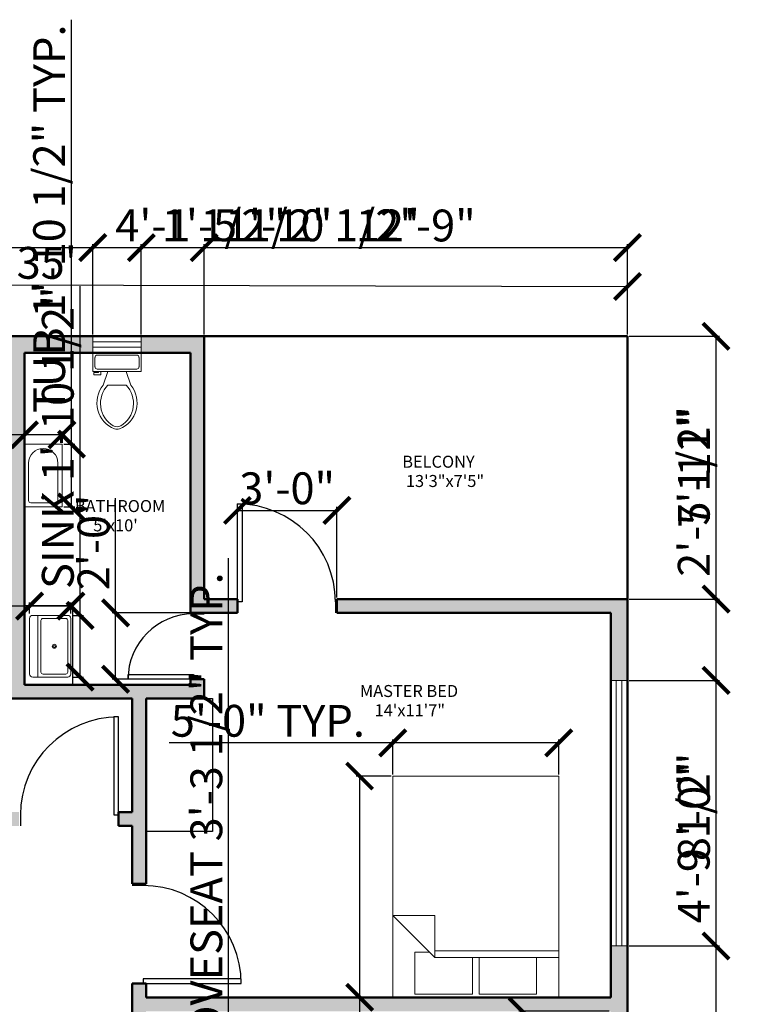
# Model space of a CAD drawing. Units: inches. Extents: x 3147 to 3847, y 1414 to 2207.
# Tile 7 of 7: x 3550 to 3812, y 1852 to 2207. Entities that reach past the tile are written whole.
import ezdxf

# ---------------------------------------------------------------- set-up
doc = ezdxf.new("R2010")
doc.units = ezdxf.units.IN
for name, color, linetype, lineweight in [('A-ANNO-DIMS', 2, 'Continuous', 18), ('A-AREA-IDEN', 7, 'Continuous', 18), ('A-DOOR', 3, 'Continuous', 25), ('A-FLOR-CASE', 32, 'Continuous', 25), ('A-FLOR-FIXT', 9, 'Continuous', 18), ('A-FURN', 8, 'Continuous', 18), ('A-GLAZ', 4, 'Continuous', 18), ('A-WALL', 7, 'Continuous', 50)]:
    doc.layers.add(name, color=color, linetype=linetype, lineweight=lineweight)
doc.layers.add('A-WALL-PATT', color=18, linetype='Continuous', lineweight=13, true_color=0x000000)
doc.styles.get("Standard").update_dxf_attribs({"font": 'arial.ttf'})
doc.dimstyles.new('ISO-25', dxfattribs={"dimtxt": 11.5, "dimasz": 9.5, "dimexe": 1.25, "dimexo": 0.625, "dimtad": 1, "dimdec": 0, "dimlunit": 3, "dimtxsty": 'Standard', "dimblk": 'ARCHTICK', "dimcen": 2.5, "dimadec": 0, "dimazin": 0, "dimtfac": 1, "dimtdec": 0, "dimtmove": 0, "dimatfit": 3, "dimfxl": 1, "dimarcsym": 0})

# ---------------------------------------------------------------- blocks, each defined once
blk = doc.blocks.new('*U6')
for p, q in [((0, 0), (0, -100)), ((900, 0), (900, -100))]:
    blk.add_line(p, q)
blk.add_lwpolyline([(0, 0), (0, 900), (43.75, 900), (43.75, 0)], close=True)
blk.add_arc((0, 0), 900, 0, 90)
blk = doc.blocks.new('*U5')
for p, q in [((0, 0), (0, -100)), ((-900, 0), (-900, -100))]:
    blk.add_line(p, q)
blk.add_lwpolyline([(0, 0), (0, 900), (-43.75, 900), (-43.75, 0)], close=True)
blk.add_arc((0, 0), 900, 90, 180)
blk = doc.blocks.new('*U7')
for p, q in [((0, 0), (0, -100)), ((600, 0), (600, -100))]:
    blk.add_line(p, q)
blk.add_lwpolyline([(0, 0), (0, 600), (43.75, 600), (43.75, 0)], close=True)
blk.add_arc((0, 0), 600, 0, 90)
blk = doc.blocks.new('Bed - Queen')
for p, q in [((0, -80.00003), (0, 0)), ((0, 0), (59.99999, 0)), ((59.99999, 0), (59.99999, -80.00003)), ((7.99999, -1.2), (28.79998, -1.2)), ((7.99999, -14.4), (7.99999, -1.2)), ((28.79998, -1.2), (28.79998, -14.4)), ((31.19999, -1.2), (51.99999, -1.2)), ((31.19999, -14.4), (31.19999, -1.2)), ((51.99999, -1.2), (51.99999, -16.4)), ((0, -14.4), (44.8, -14.4)), ((44.8, -16.8), (0, -16.8)), ((59.99999, -29.6), (44.8, -14.4)), ((44.8, -14.4), (44.8, -29.6)), ((51.99999, -16.4), (46.79936, -16.4)), ((44.8, -29.6), (59.99999, -29.6)), ((59.99999, -80.00003), (0, -80.00003))]:
    blk.add_line(p, q)
blk = doc.blocks.new('Sink-single - 30 in top')
blk.add_line((-15, -3.999996), (15, -3.999996))
for points in [[(-13.5, 0), (13.5, 0)], [(-15, -18.499996), (-15, -1.5)], [(15, -1.5), (15, -18.499996)], [(-13.5, -17.499996), (-13.5, -6.499996)], [(-12.5, -5.499996), (12.5, -5.499996)], [(13.5, -6.499996), (13.5, -17.499996)], [(12.5, -18.499996), (-12.5, -18.499996)], [(13.5, -19.999996), (-13.5, -19.999996)]]:
    blk.add_lwpolyline(points)
for radius in [1, 0.5]:
    blk.add_circle((0, -11.999996), radius)
for centre, radius, start, end in [((-13.5, -1.5), 1.5, 90, 180), ((13.5, -1.5), 1.5, 0, 90), ((-12.5, -6.499996), 1, 90, 180), ((12.5, -6.499996), 1, 0, 90), ((-13.5, -18.499996), 1.5, 180, 270), ((-12.5, -17.499996), 1, 180, 270), ((12.5, -17.499996), 1, 270, 0), ((13.5, -18.499996), 1.5, 270, 0)]:
    blk.add_arc(centre, radius, start, end)
blk = doc.blocks.new('Toilet - top')
for p, q in [((9.5, -6), (9.5, -2)), ((-10, -8.5), (-8, -8.5)), ((-10, -9.5), (-10, -8.5)), ((-8, -8.5), (-8, -8)), ((-7, -8), (-7, -9.5)), ((-4, -8), (-6, -14)), ((4, -8), (6, -14)), ((-7, -9.5), (-10, -9.5)), ((4, -14), (-4, -14))]:
    blk.add_line(p, q)
blk.add_lwpolyline([(10.5, -8), (10.5, 0), (-10.5, 0), (-10.5, -8)], close=True)
for points in [[(-9.5, -2), (-9.5, -6)], [(8.5, -1), (-8.5, -1)], [(-8.5, -7), (8.5, -7)]]:
    blk.add_lwpolyline(points)
for centre, radius, start, end in [((-8.62, -1.88), 0.884, 81.8699, 188.1301), ((8.62, -1.88), 0.884, 351.8699, 98.1301), ((-8.62, -6.12), 0.884, 171.8699, 278.1301), ((8.62, -6.12), 0.884, 261.8699, 8.1301), ((3.52, -21.58), 12.17, 141.4691, 247.9714), ((4.2, -21.82), 11.33, 136.3677, 238.9468), ((-3.52, -21.58), 12.17, 292.0284, 38.5307), ((-4.2, -21.82), 11.33, 301.053, 43.6321), ((0, -27.88), 4, 245.7318, 294.2682), ((0, -29), 4, 254.8605, 285.1395)]:
    blk.add_arc(centre, radius, start, end)
blk = doc.blocks.new('Bath Tub - 26 x 60 in.')
for p, q in [((8, -18), (10, -18)), ((9, -17), (9, -19))]:
    blk.add_line(p, q)
blk.add_lwpolyline([(0, -36), (0, 0), (60, 0), (60, -36)], close=True)
for points in [[(4, -30), (4, -6)], [(6, -4), (42, -4)], [(42, -32), (6, -32)]]:
    blk.add_lwpolyline(points)
for radius in [1.5, 1]:
    blk.add_circle((9, -18), radius)
for centre, radius, start, end in [((5.75, -5.75), 1.77, 81.8699, 188.1301), ((42, -18), 14, 270, 90), ((5.75, -30.25), 1.77, 171.8699, 278.1301)]:
    blk.add_arc(centre, radius, start, end)
blk = doc.blocks.new('_ArchTick')
at = {"color": 0, "linetype": 'ByBlock', "const_width": 0.15}
blk.add_lwpolyline([(-0.5, -0.5), (0.5, 0.5)], dxfattribs=at)
blk = doc.blocks.new('*D23')
at = {"layer": 'A-ANNO-DIMS', "color": 0, "lineweight": -2, "transparency": 16777216}
for p, q in [((3349.77, 2094.75), (3349.81, 2113.37)), ((3349.81, 2112.12), (3769.81, 2111.04)), ((3769.77, 2093.67), (3769.81, 2112.29))]:
    blk.add_line(p, q, dxfattribs=at)
at = {"layer": 'Defpoints', "color": 0, "transparency": 16777216}
for p in [(3769.81, 2111.04), (3349.76, 2094.13), (3769.76, 2093.05)]:
    blk.add_point(p, dxfattribs=at)
at = {"layer": 'A-ANNO-DIMS', "color": 0, "lineweight": -2, "transparency": 16777216, "xscale": 9.5, "yscale": 9.5, "zscale": 9.5}
for p, rotation in [((3349.81, 2112.12), 179.8528346034433), ((3769.81, 2111.04), 359.8528346034433)]:
    blk.add_blockref('_ArchTick', p, dxfattribs=dict(at, rotation=rotation))
at = {"layer": 'A-ANNO-DIMS', "color": 0, "transparency": 16777216, "insert": (3559.83, 2118.08), "char_height": 11.5, "attachment_point": 5, "rotation": 359.8528}
blk.add_mtext("35'", dxfattribs=at)
blk = doc.blocks.new('*D29')
at = {"layer": 'A-ANNO-DIMS', "color": 0, "lineweight": -2, "transparency": 16777216}
for p, q in [((3568.76, 2054.03), (3568.76, 2207.49)), ((3565.99, 2054.03), (3570.01, 2054.03)), ((3568.76, 2031.36), (3568.76, 2054.03)), ((3565.99, 2031.36), (3570.01, 2031.36))]:
    blk.add_line(p, q, dxfattribs=at)
at = {"layer": 'Defpoints', "color": 0, "transparency": 16777216}
for p in [(3565.36, 2054.03), (3568.76, 2054.03), (3565.36, 2031.36)]:
    blk.add_point(p, dxfattribs=at)
at = {"layer": 'A-ANNO-DIMS', "color": 0, "lineweight": -2, "transparency": 16777216, "xscale": 9.5, "yscale": 9.5, "zscale": 9.5}
for p, rotation in [((3568.76, 2054.03), 90), ((3568.76, 2031.36), 270)]:
    blk.add_blockref('_ArchTick', p, dxfattribs=dict(at, rotation=rotation))
at = {"layer": 'A-ANNO-DIMS', "color": 0, "transparency": 16777216, "insert": (3562.19, 2135.51), "char_height": 11.5, "attachment_point": 5, "rotation": 90}
blk.add_mtext('TUB 1\'-10 1/2" TYP.', dxfattribs=at)
blk = doc.blocks.new('*D30')
at = {"layer": 'A-ANNO-DIMS', "color": 0, "lineweight": -2, "transparency": 16777216}
for p, q in [((3551.76, 2057.43), (3445.2, 2057.43)), ((3551.76, 2054.65), (3551.76, 2058.68)), ((3565.36, 2057.43), (3551.76, 2057.43)), ((3565.36, 2054.65), (3565.36, 2058.68))]:
    blk.add_line(p, q, dxfattribs=at)
at = {"layer": 'Defpoints', "color": 0, "transparency": 16777216}
for p in [(3551.76, 2057.43), (3551.76, 2054.03), (3565.36, 2054.03)]:
    blk.add_point(p, dxfattribs=at)
at = {"layer": 'A-ANNO-DIMS', "color": 0, "lineweight": -2, "transparency": 16777216, "xscale": 9.5, "yscale": 9.5, "zscale": 9.5, "rotation": 180}
blk.add_blockref('_ArchTick', (3551.76, 2057.43), dxfattribs=at)
at = {"layer": 'A-ANNO-DIMS', "color": 0, "lineweight": -2, "transparency": 16777216, "xscale": 9.5, "yscale": 9.5, "zscale": 9.5}
blk.add_blockref('_ArchTick', (3565.36, 2057.43), dxfattribs=at)
at = {"layer": 'A-ANNO-DIMS', "color": 0, "transparency": 16777216, "insert": (3493.73, 2064), "char_height": 11.5, "attachment_point": 5}
blk.add_mtext('1\'-1 1/2" TYP.', dxfattribs=at)
blk = doc.blocks.new('*D33')
at = {"layer": 'A-ANNO-DIMS', "color": 0, "lineweight": -2, "transparency": 16777216}
for p, q in [((3684.32, 1934.05), (3671.7, 1934.05)), ((3672.95, 1934.05), (3672.95, 1854.05)), ((3684.32, 1854.05), (3671.7, 1854.05)), ((3672.95, 1854.05), (3672.95, 1736.21))]:
    blk.add_line(p, q, dxfattribs=at)
at = {"layer": 'Defpoints', "color": 0, "transparency": 16777216}
for p in [(3684.95, 1934.05), (3672.95, 1854.05), (3684.95, 1854.05)]:
    blk.add_point(p, dxfattribs=at)
at = {"layer": 'A-ANNO-DIMS', "color": 0, "lineweight": -2, "transparency": 16777216, "xscale": 9.5, "yscale": 9.5, "zscale": 9.5}
for p, rotation in [((3672.95, 1934.05), 90), ((3672.95, 1854.05), 270)]:
    blk.add_blockref('_ArchTick', p, dxfattribs=dict(at, rotation=rotation))
at = {"layer": 'A-ANNO-DIMS', "color": 0, "transparency": 16777216, "insert": (3666.45, 1790.38), "char_height": 11.5, "attachment_point": 5, "rotation": 90}
blk.add_mtext('BED 6\'-8" TYP.', dxfattribs=at)
blk = doc.blocks.new('*D34')
at = {"layer": 'A-ANNO-DIMS', "color": 0, "lineweight": -2, "transparency": 16777216}
for p, q in [((3684.95, 1934.67), (3684.95, 1947.3)), ((3744.95, 1934.67), (3744.95, 1947.3)), ((3684.95, 1946.05), (3604.1, 1946.05)), ((3744.95, 1946.05), (3684.95, 1946.05))]:
    blk.add_line(p, q, dxfattribs=at)
at = {"layer": 'Defpoints', "color": 0, "transparency": 16777216}
for p in [(3684.95, 1946.05), (3684.95, 1934.05), (3744.95, 1934.05)]:
    blk.add_point(p, dxfattribs=at)
at = {"layer": 'A-ANNO-DIMS', "color": 0, "lineweight": -2, "transparency": 16777216, "xscale": 9.5, "yscale": 9.5, "zscale": 9.5, "rotation": 180}
blk.add_blockref('_ArchTick', (3684.95, 1946.05), dxfattribs=at)
at = {"layer": 'A-ANNO-DIMS', "color": 0, "lineweight": -2, "transparency": 16777216, "xscale": 9.5, "yscale": 9.5, "zscale": 9.5}
blk.add_blockref('_ArchTick', (3744.95, 1946.05), dxfattribs=at)
at = {"layer": 'A-ANNO-DIMS', "color": 0, "transparency": 16777216, "insert": (3639.78, 1952.55), "char_height": 11.5, "attachment_point": 5}
blk.add_mtext('5\'-0" TYP.', dxfattribs=at)
blk = doc.blocks.new('*D37')
at = {"layer": 'A-ANNO-DIMS', "color": 0, "lineweight": -2, "transparency": 16777216}
for p, q in [((3625.6, 1816.38), (3625.6, 2012.8)), ((3620.32, 1816.38), (3626.85, 1816.38)), ((3625.6, 1777.02), (3625.6, 1816.38)), ((3620.32, 1777.02), (3626.85, 1777.02))]:
    blk.add_line(p, q, dxfattribs=at)
at = {"layer": 'Defpoints', "color": 0, "transparency": 16777216}
for p in [(3619.7, 1816.38), (3625.6, 1816.38), (3619.7, 1777.02)]:
    blk.add_point(p, dxfattribs=at)
at = {"layer": 'A-ANNO-DIMS', "color": 0, "lineweight": -2, "transparency": 16777216, "xscale": 9.5, "yscale": 9.5, "zscale": 9.5}
for p, rotation in [((3625.6, 1816.38), 90), ((3625.6, 1777.02), 270)]:
    blk.add_blockref('_ArchTick', p, dxfattribs=dict(at, rotation=rotation))
at = {"layer": 'A-ANNO-DIMS', "color": 0, "transparency": 16777216, "insert": (3619.02, 1919.34), "char_height": 11.5, "attachment_point": 5, "rotation": 90}
blk.add_mtext('LOVESEAT 3\'-3 1/2" TYP.', dxfattribs=at)
blk = doc.blocks.new('*D47')
at = {"layer": 'A-ANNO-DIMS', "color": 0, "lineweight": -2, "transparency": 16777216}
for p, q in [((3571.89, 1992.16), (3571.89, 2111.11)), ((3569.17, 1992.16), (3573.14, 1992.16)), ((3571.89, 1969.81), (3571.89, 1992.16)), ((3569.17, 1969.81), (3573.14, 1969.81))]:
    blk.add_line(p, q, dxfattribs=at)
at = {"layer": 'Defpoints', "color": 0, "transparency": 16777216}
for p in [(3568.54, 1992.16), (3571.89, 1992.16), (3568.54, 1969.81)]:
    blk.add_point(p, dxfattribs=at)
at = {"layer": 'A-ANNO-DIMS', "color": 0, "lineweight": -2, "transparency": 16777216, "xscale": 9.5, "yscale": 9.5, "zscale": 9.5}
for p, rotation in [((3571.89, 1992.16), 90), ((3571.89, 1969.81), 270)]:
    blk.add_blockref('_ArchTick', p, dxfattribs=dict(at, rotation=rotation))
at = {"layer": 'A-ANNO-DIMS', "color": 0, "transparency": 16777216, "insert": (3565.32, 2056.38), "char_height": 11.5, "attachment_point": 5, "rotation": 90}
blk.add_mtext('SINK 1\'-10 1/2"', dxfattribs=at)
blk = doc.blocks.new('*D48')
at = {"layer": 'A-ANNO-DIMS', "color": 0, "lineweight": -2, "transparency": 16777216}
for p, q in [((3553.64, 1995.51), (3513.41, 1995.51)), ((3553.64, 1992.78), (3553.64, 1996.76)), ((3568.54, 1995.51), (3553.64, 1995.51)), ((3568.54, 1992.78), (3568.54, 1996.76))]:
    blk.add_line(p, q, dxfattribs=at)
at = {"layer": 'Defpoints', "color": 0, "transparency": 16777216}
for p in [(3553.64, 1995.51), (3553.64, 1992.16), (3568.54, 1992.16)]:
    blk.add_point(p, dxfattribs=at)
at = {"layer": 'A-ANNO-DIMS', "color": 0, "lineweight": -2, "transparency": 16777216, "xscale": 9.5, "yscale": 9.5, "zscale": 9.5, "rotation": 180}
blk.add_blockref('_ArchTick', (3553.64, 1995.51), dxfattribs=at)
at = {"layer": 'A-ANNO-DIMS', "color": 0, "lineweight": -2, "transparency": 16777216, "xscale": 9.5, "yscale": 9.5, "zscale": 9.5}
blk.add_blockref('_ArchTick', (3568.54, 1995.51), dxfattribs=at)
at = {"layer": 'A-ANNO-DIMS', "color": 0, "transparency": 16777216, "insert": (3528.78, 2002.01), "char_height": 11.5, "attachment_point": 5}
blk.add_mtext('1\'-3"', dxfattribs=at)
blk = doc.blocks.new('*D58')
at = {"layer": 'A-ANNO-DIMS', "color": 0, "lineweight": -2, "transparency": 16777216}
for p, q in [((3801.81, 1872.64), (3801.81, 1941.22)), ((3770.39, 1872.64), (3803.06, 1872.64)), ((3801.81, 1815.24), (3801.81, 1872.64)), ((3770.39, 1815.24), (3803.06, 1815.24))]:
    blk.add_line(p, q, dxfattribs=at)
at = {"layer": 'Defpoints', "color": 0, "transparency": 16777216}
for p in [(3769.76, 1872.64), (3801.81, 1872.64), (3769.76, 1815.24)]:
    blk.add_point(p, dxfattribs=at)
at = {"layer": 'A-ANNO-DIMS', "color": 0, "lineweight": -2, "transparency": 16777216, "xscale": 9.5, "yscale": 9.5, "zscale": 9.5}
for p, rotation in [((3801.81, 1872.64), 90), ((3801.81, 1815.24), 270)]:
    blk.add_blockref('_ArchTick', p, dxfattribs=dict(at, rotation=rotation))
at = {"layer": 'A-ANNO-DIMS', "color": 0, "transparency": 16777216, "insert": (3795.24, 1911.68), "char_height": 11.5, "attachment_point": 5, "rotation": 90}
blk.add_mtext('4\'-9 1/2"', dxfattribs=at)
blk = doc.blocks.new('*D59')
at = {"layer": 'A-ANNO-DIMS', "color": 0, "lineweight": -2, "transparency": 16777216}
for p, q in [((3770.39, 1968.64), (3803.06, 1968.64)), ((3801.81, 1872.64), (3801.81, 1968.64)), ((3770.39, 1872.64), (3803.06, 1872.64))]:
    blk.add_line(p, q, dxfattribs=at)
at = {"layer": 'Defpoints', "color": 0, "transparency": 16777216}
for p in [(3769.76, 1968.64), (3801.81, 1968.64), (3769.76, 1872.64)]:
    blk.add_point(p, dxfattribs=at)
at = {"layer": 'A-ANNO-DIMS', "color": 0, "lineweight": -2, "transparency": 16777216, "xscale": 9.5, "yscale": 9.5, "zscale": 9.5}
for p, rotation in [((3801.81, 1968.64), 90), ((3801.81, 1872.64), 270)]:
    blk.add_blockref('_ArchTick', p, dxfattribs=dict(at, rotation=rotation))
at = {"layer": 'A-ANNO-DIMS', "color": 0, "transparency": 16777216, "insert": (3795.32, 1920.64), "char_height": 11.5, "attachment_point": 5, "rotation": 90}
blk.add_mtext('8\'-0"', dxfattribs=at)
blk = doc.blocks.new('*D60')
at = {"layer": 'A-ANNO-DIMS', "color": 0, "lineweight": -2, "transparency": 16777216}
for p, q in [((3801.81, 1998.05), (3801.81, 2066.36)), ((3770.39, 1998.05), (3803.06, 1998.05)), ((3801.81, 1968.64), (3801.81, 1998.05)), ((3770.39, 1968.64), (3803.06, 1968.64))]:
    blk.add_line(p, q, dxfattribs=at)
at = {"layer": 'Defpoints', "color": 0, "transparency": 16777216}
for p in [(3769.76, 1998.05), (3801.81, 1998.05), (3769.76, 1968.64)]:
    blk.add_point(p, dxfattribs=at)
at = {"layer": 'A-ANNO-DIMS', "color": 0, "lineweight": -2, "transparency": 16777216, "xscale": 9.5, "yscale": 9.5, "zscale": 9.5}
for p, rotation in [((3801.81, 1998.05), 90), ((3801.81, 1968.64), 270)]:
    blk.add_blockref('_ArchTick', p, dxfattribs=dict(at, rotation=rotation))
at = {"layer": 'A-ANNO-DIMS', "color": 0, "transparency": 16777216, "insert": (3795.24, 2036.96), "char_height": 11.5, "attachment_point": 5, "rotation": 90}
blk.add_mtext('2\'-5 1/2"', dxfattribs=at)
blk = doc.blocks.new('*D61')
at = {"layer": 'A-ANNO-DIMS', "color": 0, "lineweight": -2, "transparency": 16777216}
for p, q in [((3770.39, 2093.05), (3803.06, 2093.05)), ((3801.81, 1998.05), (3801.81, 2093.05)), ((3770.39, 1998.05), (3803.06, 1998.05))]:
    blk.add_line(p, q, dxfattribs=at)
at = {"layer": 'Defpoints', "color": 0, "transparency": 16777216}
for p in [(3769.76, 2093.05), (3801.81, 2093.05), (3769.76, 1998.05)]:
    blk.add_point(p, dxfattribs=at)
at = {"layer": 'A-ANNO-DIMS', "color": 0, "lineweight": -2, "transparency": 16777216, "xscale": 9.5, "yscale": 9.5, "zscale": 9.5}
for p, rotation in [((3801.81, 2093.05), 90), ((3801.81, 1998.05), 270)]:
    blk.add_blockref('_ArchTick', p, dxfattribs=dict(at, rotation=rotation))
at = {"layer": 'A-ANNO-DIMS', "color": 0, "transparency": 16777216, "insert": (3795.42, 2045.55), "char_height": 11.5, "attachment_point": 5, "rotation": 90}
blk.add_mtext('7\'-11"', dxfattribs=at)
blk = doc.blocks.new('*D65')
at = {"layer": 'A-ANNO-DIMS', "color": 0, "lineweight": -2, "transparency": 16777216}
for p, q in [((3527.03, 2093.67), (3527.03, 2126.35)), ((3527.03, 2125.1), (3576.44, 2125.1)), ((3576.44, 2093.67), (3576.44, 2126.35)), ((3576.44, 2125.1), (3645.01, 2125.1))]:
    blk.add_line(p, q, dxfattribs=at)
at = {"layer": 'Defpoints', "color": 0, "transparency": 16777216}
for p in [(3576.44, 2125.1), (3527.03, 2093.05), (3576.44, 2093.05)]:
    blk.add_point(p, dxfattribs=at)
at = {"layer": 'A-ANNO-DIMS', "color": 0, "lineweight": -2, "transparency": 16777216, "xscale": 9.5, "yscale": 9.5, "zscale": 9.5, "rotation": 180}
blk.add_blockref('_ArchTick', (3527.03, 2125.1), dxfattribs=at)
at = {"layer": 'A-ANNO-DIMS', "color": 0, "lineweight": -2, "transparency": 16777216, "xscale": 9.5, "yscale": 9.5, "zscale": 9.5}
blk.add_blockref('_ArchTick', (3576.44, 2125.1), dxfattribs=at)
at = {"layer": 'A-ANNO-DIMS', "color": 0, "transparency": 16777216, "insert": (3615.48, 2131.67), "char_height": 11.5, "attachment_point": 5}
blk.add_mtext('4\'-1 1/2"', dxfattribs=at)
blk = doc.blocks.new('*D66')
at = {"layer": 'A-ANNO-DIMS', "color": 0, "lineweight": -2, "transparency": 16777216}
for p, q in [((3576.44, 2093.67), (3576.44, 2126.35)), ((3576.44, 2125.1), (3594.02, 2125.1)), ((3594.02, 2093.67), (3594.02, 2126.35)), ((3594.02, 2125.1), (3661.06, 2125.1))]:
    blk.add_line(p, q, dxfattribs=at)
at = {"layer": 'Defpoints', "color": 0, "transparency": 16777216}
for p in [(3594.02, 2125.1), (3576.44, 2093.05), (3594.02, 2093.05)]:
    blk.add_point(p, dxfattribs=at)
at = {"layer": 'A-ANNO-DIMS', "color": 0, "lineweight": -2, "transparency": 16777216, "xscale": 9.5, "yscale": 9.5, "zscale": 9.5, "rotation": 180}
blk.add_blockref('_ArchTick', (3576.44, 2125.1), dxfattribs=at)
at = {"layer": 'A-ANNO-DIMS', "color": 0, "lineweight": -2, "transparency": 16777216, "xscale": 9.5, "yscale": 9.5, "zscale": 9.5}
blk.add_blockref('_ArchTick', (3594.02, 2125.1), dxfattribs=at)
at = {"layer": 'A-ANNO-DIMS', "color": 0, "transparency": 16777216, "insert": (3632.29, 2131.67), "char_height": 11.5, "attachment_point": 5}
blk.add_mtext('1\'-5 1/2"', dxfattribs=at)
blk = doc.blocks.new('*D67')
at = {"layer": 'A-ANNO-DIMS', "color": 0, "lineweight": -2, "transparency": 16777216}
for p, q in [((3594.02, 2093.67), (3594.02, 2126.35)), ((3594.02, 2125.1), (3616.76, 2125.1)), ((3616.76, 2093.67), (3616.76, 2126.35)), ((3616.76, 2125.1), (3692.73, 2125.1))]:
    blk.add_line(p, q, dxfattribs=at)
at = {"layer": 'Defpoints', "color": 0, "transparency": 16777216}
for p in [(3616.76, 2125.1), (3594.02, 2093.05), (3616.76, 2093.05)]:
    blk.add_point(p, dxfattribs=at)
at = {"layer": 'A-ANNO-DIMS', "color": 0, "lineweight": -2, "transparency": 16777216, "xscale": 9.5, "yscale": 9.5, "zscale": 9.5, "rotation": 180}
blk.add_blockref('_ArchTick', (3594.02, 2125.1), dxfattribs=at)
at = {"layer": 'A-ANNO-DIMS', "color": 0, "lineweight": -2, "transparency": 16777216, "xscale": 9.5, "yscale": 9.5, "zscale": 9.5}
blk.add_blockref('_ArchTick', (3616.76, 2125.1), dxfattribs=at)
at = {"layer": 'A-ANNO-DIMS', "color": 0, "transparency": 16777216, "insert": (3659.5, 2131.67), "char_height": 11.5, "attachment_point": 5}
blk.add_mtext('1\'-10 1/2"', dxfattribs=at)
blk = doc.blocks.new('*D68')
at = {"layer": 'A-ANNO-DIMS', "color": 0, "lineweight": -2, "transparency": 16777216}
for p, q in [((3616.76, 2093.67), (3616.76, 2126.35)), ((3616.76, 2125.1), (3769.76, 2125.1)), ((3769.76, 2093.67), (3769.76, 2126.35))]:
    blk.add_line(p, q, dxfattribs=at)
at = {"layer": 'Defpoints', "color": 0, "transparency": 16777216}
for p in [(3769.76, 2125.1), (3616.76, 2093.05), (3769.76, 2093.05)]:
    blk.add_point(p, dxfattribs=at)
at = {"layer": 'A-ANNO-DIMS', "color": 0, "lineweight": -2, "transparency": 16777216, "xscale": 9.5, "yscale": 9.5, "zscale": 9.5, "rotation": 180}
blk.add_blockref('_ArchTick', (3616.76, 2125.1), dxfattribs=at)
at = {"layer": 'A-ANNO-DIMS', "color": 0, "lineweight": -2, "transparency": 16777216, "xscale": 9.5, "yscale": 9.5, "zscale": 9.5}
blk.add_blockref('_ArchTick', (3769.76, 2125.1), dxfattribs=at)
at = {"layer": 'A-ANNO-DIMS', "color": 0, "transparency": 16777216, "insert": (3693.26, 2131.6), "char_height": 11.5, "attachment_point": 5}
blk.add_mtext('12\'-9"', dxfattribs=at)
blk = doc.blocks.new('*D84')
at = {"layer": 'A-ANNO-DIMS', "color": 0, "lineweight": -2, "transparency": 16777216}
for p, q in [((3628.76, 1998.67), (3628.76, 2031.35)), ((3628.76, 2030.1), (3664.76, 2030.1)), ((3664.76, 1998.67), (3664.76, 2031.35))]:
    blk.add_line(p, q, dxfattribs=at)
at = {"layer": 'Defpoints', "color": 0, "transparency": 16777216}
for p in [(3664.76, 2030.1), (3628.76, 1998.05), (3664.76, 1998.05)]:
    blk.add_point(p, dxfattribs=at)
at = {"layer": 'A-ANNO-DIMS', "color": 0, "lineweight": -2, "transparency": 16777216, "xscale": 9.5, "yscale": 9.5, "zscale": 9.5, "rotation": 180}
blk.add_blockref('_ArchTick', (3628.76, 2030.1), dxfattribs=at)
at = {"layer": 'A-ANNO-DIMS', "color": 0, "lineweight": -2, "transparency": 16777216, "xscale": 9.5, "yscale": 9.5, "zscale": 9.5}
blk.add_blockref('_ArchTick', (3664.76, 2030.1), dxfattribs=at)
at = {"layer": 'A-ANNO-DIMS', "color": 0, "transparency": 16777216, "insert": (3646.76, 2036.6), "char_height": 11.5, "attachment_point": 5}
blk.add_mtext('3\'-0"', dxfattribs=at)
blk = doc.blocks.new('*D85')
at = {"layer": 'A-ANNO-DIMS', "color": 0, "lineweight": -2, "transparency": 16777216}
for p, q in [((3584.71, 1993.05), (3584.71, 2034.57)), ((3616.14, 1993.05), (3583.46, 1993.05)), ((3584.71, 1969.05), (3584.71, 1993.05)), ((3616.14, 1969.05), (3583.46, 1969.05))]:
    blk.add_line(p, q, dxfattribs=at)
at = {"layer": 'Defpoints', "color": 0, "transparency": 16777216}
for p in [(3584.71, 1993.05), (3616.76, 1993.05), (3616.76, 1969.05)]:
    blk.add_point(p, dxfattribs=at)
at = {"layer": 'A-ANNO-DIMS', "color": 0, "lineweight": -2, "transparency": 16777216, "xscale": 9.5, "yscale": 9.5, "zscale": 9.5}
for p, rotation in [((3584.71, 1993.05), 90), ((3584.71, 1969.05), 270)]:
    blk.add_blockref('_ArchTick', p, dxfattribs=dict(at, rotation=rotation))
at = {"layer": 'A-ANNO-DIMS', "color": 0, "transparency": 16777216, "insert": (3578.22, 2018.56), "char_height": 11.5, "attachment_point": 5, "rotation": 90}
blk.add_mtext('2\'-0"', dxfattribs=at)
blk = doc.blocks.new('*D88')
at = {"layer": 'A-ANNO-DIMS', "color": 0, "lineweight": -2, "transparency": 16777216}
for p, q in [((3763.14, 1849.05), (3730.46, 1849.05)), ((3731.71, 1718.05), (3731.71, 1849.05)), ((3763.14, 1718.05), (3730.46, 1718.05))]:
    blk.add_line(p, q, dxfattribs=at)
at = {"layer": 'Defpoints', "color": 0, "transparency": 16777216}
for p in [(3731.71, 1849.05), (3763.76, 1849.05), (3763.76, 1718.05)]:
    blk.add_point(p, dxfattribs=at)
at = {"layer": 'A-ANNO-DIMS', "color": 0, "lineweight": -2, "transparency": 16777216, "xscale": 9.5, "yscale": 9.5, "zscale": 9.5}
for p, rotation in [((3731.71, 1849.05), 90), ((3731.71, 1718.05), 270)]:
    blk.add_blockref('_ArchTick', p, dxfattribs=dict(at, rotation=rotation))
at = {"layer": 'A-ANNO-DIMS', "color": 0, "transparency": 16777216, "insert": (3725.22, 1783.55), "char_height": 11.5, "attachment_point": 5, "rotation": 90}
blk.add_mtext('10\'-11"', dxfattribs=at)

msp = doc.modelspace()

# ---------------------------------------------------------------- hatches: boundary and pattern name
at = {"layer": 'A-WALL-PATT'}
h = msp.add_hatch(color=256, dxfattribs=at)
h.dxf.hatch_style = 1
h.paths.add_polyline_path([(3616.76, 2093.05), (3594.02, 2093.05), (3594.02, 2087.05), (3611.76, 2087.05), (3611.76, 1993.05), (3616.76, 1993.05), (3628.76, 1993.05), (3628.76, 1996.99), (3628.76, 1998.05), (3616.76, 1998.05), (3616.76, 2087.05)])
h.paths.add_polyline_path([(3576.44, 2093.05), (3527.03, 2093.05), (3527.03, 2087.05), (3546.76, 2087.05), (3546.76, 1962.05), (3551.76, 1962.05), (3590.76, 1962.05), (3590.76, 1921.05), (3585.76, 1921.05), (3585.76, 1916.05), (3590.76, 1916.05), (3590.76, 1895.05), (3595.76, 1895.05), (3595.76, 1962.05), (3611.76, 1962.05), (3616.76, 1962.05), (3616.76, 1969.05), (3611.76, 1969.05), (3611.76, 1967.05), (3551.76, 1967.05), (3551.76, 2087.05), (3576.44, 2087.05)])
h.paths.add_polyline_path([(3455.03, 2093.05), (3408.76, 2093.05), (3408.76, 2087.05), (3408.76, 2046.06), (3413.76, 2046.06), (3413.76, 2087.05), (3455.03, 2087.05)])
h.paths.add_polyline_path([(3355.76, 2008.05), (3408.76, 2008.05), (3408.76, 2004.83), (3413.76, 2004.83), (3413.76, 2008.05), (3413.76, 2013.05), (3413.76, 2016.06), (3408.76, 2016.06), (3408.76, 2013.05), (3355.76, 2013.05), (3349.76, 2013.05), (3349.76, 1973.71), (3355.76, 1973.71)])
h.paths.add_polyline_path([(3413.76, 1974.83), (3408.76, 1974.83), (3408.76, 1943.05), (3355.76, 1943.05), (3355.76, 1949.71), (3349.76, 1949.71), (3349.76, 1897.34), (3355.76, 1897.34), (3355.76, 1938.05), (3408.76, 1938.05), (3408.76, 1934.63), (3413.76, 1934.63), (3413.76, 1938.05), (3505.76, 1938.05), (3505.76, 1916.05), (3533.76, 1916.05), (3533.76, 1904.63), (3533.76, 1831.83), (3538.76, 1831.83), (3538.76, 1904.63), (3538.76, 1916.05), (3546.76, 1916.05), (3549.76, 1916.05), (3549.76, 1921.05), (3546.76, 1921.05), (3510.76, 1921.05), (3510.76, 1938.05), (3510.76, 1943.05), (3413.76, 1943.05)])
h.paths.add_polyline_path([(3413.76, 1904.63), (3408.76, 1904.63), (3408.76, 1870.05), (3355.76, 1870.05), (3355.76, 1873.34), (3349.76, 1873.34), (3349.76, 1865.05), (3355.76, 1865.05), (3408.76, 1865.05), (3408.76, 1863.11), (3409.83, 1863.11), (3413.76, 1863.11)], flags=17)
h.paths.add_polyline_path([(3538.76, 1795.83), (3533.76, 1795.83), (3533.76, 1794.05), (3413.76, 1794.05), (3413.76, 1833.11), (3408.76, 1833.11), (3408.76, 1794.05), (3355.76, 1794.05), (3349.76, 1794.05), (3349.76, 1776.88), (3355.76, 1776.88), (3355.76, 1789.05), (3413.76, 1789.05), (3475.76, 1789.05), (3475.76, 1731.91), (3480.76, 1731.91), (3480.76, 1789.05), (3538.76, 1789.05)])
h.paths.add_polyline_path([(3432.14, 1733.05), (3413.76, 1733.05), (3355.76, 1733.05), (3355.76, 1740.88), (3349.76, 1740.88), (3349.76, 1720.47), (3355.76, 1720.47), (3355.76, 1729.05), (3413.76, 1729.05), (3432.14, 1729.05)])
h.paths.add_polyline_path([(3480.76, 1695.91), (3476.83, 1695.91), (3475.76, 1695.91), (3475.76, 1693.05), (3413.76, 1693.05), (3355.76, 1693.05), (3355.76, 1696.47), (3349.76, 1696.47), (3349.76, 1671.27), (3355.76, 1671.27), (3355.76, 1688.05), (3413.76, 1688.05), (3415.76, 1688.05), (3415.76, 1673.71), (3420.76, 1673.71), (3420.76, 1688.05), (3480.76, 1688.05)])
h.paths.add_polyline_path([(3420.76, 1643.71), (3415.76, 1643.71), (3415.76, 1642.05), (3413.76, 1642.05), (3355.76, 1642.05), (3355.76, 1647.27), (3349.76, 1647.27), (3349.76, 1598.35), (3355.76, 1598.35), (3355.76, 1637.05), (3401.76, 1637.05), (3401.76, 1634.26), (3406.76, 1634.26), (3406.76, 1637.05), (3413.76, 1637.05), (3420.76, 1637.05)])
h.paths.add_polyline_path([(3406.76, 1604.26), (3401.76, 1604.26), (3401.76, 1572.05), (3355.76, 1572.05), (3355.76, 1574.35), (3349.76, 1574.35), (3349.76, 1553.05), (3349.76, 1495.05), (3371.89, 1495.05), (3371.89, 1501.05), (3355.76, 1501.05), (3355.76, 1559.05), (3355.76, 1567.05), (3406.76, 1567.05), (3406.76, 1572.05)])
h.paths.add_polyline_path([(3534.41, 1501.05), (3419.89, 1501.05), (3419.89, 1495.05), (3534.41, 1495.05)])
h.paths.add_polyline_path([(3769.76, 1509.48), (3763.76, 1509.48), (3763.76, 1501.05), (3600.76, 1501.05), (3600.76, 1548.51), (3595.76, 1548.51), (3595.76, 1501.05), (3582.41, 1501.05), (3582.41, 1495.05), (3769.76, 1495.05)])
h.paths.add_polyline_path([(3769.76, 1645.82), (3763.76, 1645.82), (3763.76, 1593.05), (3664.76, 1593.05), (3619.76, 1593.05), (3619.76, 1674.05), (3614.76, 1674.05), (3614.76, 1593.05), (3595.76, 1593.05), (3595.76, 1584.51), (3600.76, 1584.51), (3600.76, 1588.05), (3619.76, 1588.05), (3664.76, 1588.05), (3763.76, 1588.05), (3763.76, 1569.48), (3769.76, 1569.48)])
h.paths.add_polyline_path([(3769.76, 1731.24), (3763.76, 1731.24), (3763.76, 1718.05), (3664.76, 1718.05), (3595.76, 1718.05), (3595.76, 1723.05), (3590.76, 1723.05), (3590.76, 1713.05), (3595.76, 1713.05), (3614.76, 1713.05), (3614.76, 1710.05), (3619.76, 1710.05), (3619.76, 1713.05), (3664.76, 1713.05), (3763.76, 1713.05), (3763.76, 1693.82), (3769.76, 1693.82)])
h.paths.add_polyline_path([(3769.76, 1872.64), (3763.76, 1872.64), (3763.76, 1854.05), (3664.76, 1854.05), (3595.76, 1854.05), (3595.76, 1859.05), (3590.76, 1859.05), (3590.76, 1759.05), (3595.76, 1759.05), (3595.76, 1849.05), (3664.76, 1849.05), (3763.76, 1849.05), (3763.76, 1815.24), (3769.76, 1815.24)])
h.paths.add_polyline_path([(3769.76, 1998.05), (3763.76, 1998.05), (3763.76, 1968.64), (3769.76, 1968.64)])
h.paths.add_polyline_path([(3763.76, 1998.05), (3664.76, 1998.05), (3664.76, 1993.05), (3763.76, 1993.05)])

# ---------------------------------------------------------------- linework, layer by layer
at = {"layer": 'A-FLOR-CASE'}
for p, q in [((3569.24, 1995.64), (3551.76, 1995.64)), ((3569.24, 1967.05), (3569.24, 1995.64)), ((3616.76, 1962.05), (3619.76, 1962.05)), ((3619.76, 1962.05), (3619.76, 1914.05)), ((3619.76, 1914.05), (3595.76, 1914.05))]:
    msp.add_line(p, q, dxfattribs=at)
at = {"layer": 'A-GLAZ'}
for p, q in [((3576.44, 2087.05), (3576.44, 2093.05)), ((3594.02, 2087.05), (3594.02, 2093.05)), ((3576.44, 2091.05), (3594.02, 2091.05)), ((3576.44, 2089.05), (3594.02, 2089.05)), ((3763.76, 1968.64), (3769.76, 1968.64)), ((3765.76, 1968.64), (3765.76, 1872.64)), ((3767.76, 1968.64), (3767.76, 1872.64)), ((3763.76, 1872.64), (3769.76, 1872.64))]:
    msp.add_line(p, q, dxfattribs=at)
at = {"layer": 'A-WALL'}
for p, q in [((3349.76, 2093.05), (3769.76, 2093.05)), ((3616.76, 2087.05), (3616.76, 2093.05)), ((3769.76, 2093.05), (3769.76, 1553.05)), ((3551.76, 1967.05), (3551.76, 2087.05)), ((3551.76, 2087.05), (3611.76, 2087.05)), ((3611.76, 1993.05), (3611.76, 2087.05)), ((3616.76, 1998.05), (3616.76, 2087.05)), ((3616.76, 1998.05), (3628.76, 1998.05)), ((3628.76, 1993.05), (3628.76, 1998.05)), ((3664.76, 1993.05), (3664.76, 1998.05)), ((3664.76, 1998.05), (3763.76, 1998.05)), ((3763.76, 1998.05), (3769.76, 1998.05)), ((3616.76, 1993.05), (3611.76, 1993.05)), ((3616.76, 1993.05), (3628.76, 1993.05)), ((3664.76, 1993.05), (3763.76, 1993.05)), ((3763.76, 1993.05), (3763.76, 1854.05)), ((3611.76, 1967.05), (3611.76, 1969.05)), ((3616.76, 1969.05), (3611.76, 1969.05)), ((3616.76, 1962.05), (3616.76, 1969.05)), ((3551.76, 1967.05), (3611.76, 1967.05)), ((3551.76, 1962.05), (3546.76, 1962.05)), ((3551.76, 1962.05), (3590.76, 1962.05)), ((3590.76, 1962.05), (3590.76, 1921.05)), ((3595.76, 1962.05), (3595.76, 1895.05)), ((3595.76, 1962.05), (3611.76, 1962.05)), ((3611.76, 1962.05), (3616.76, 1962.05)), ((3585.76, 1921.05), (3585.76, 1916.05)), ((3585.76, 1921.05), (3590.76, 1921.05)), ((3585.76, 1916.05), (3590.76, 1916.05)), ((3590.76, 1916.05), (3590.76, 1895.05)), ((3590.76, 1859.05), (3590.76, 1759.05)), ((3595.76, 1859.05), (3595.76, 1854.05))]:
    msp.add_line(p, q, dxfattribs=at)
for points in [[(3595.76, 1895.05), (3590.76, 1895.05)], [(3595.76, 1859.05), (3590.76, 1859.05)], [(3763.76, 1854.05), (3664.76, 1854.05), (3595.76, 1854.05)]]:
    msp.add_lwpolyline(points, dxfattribs=at)

# ---------------------------------------------------------------- block references
at = {"layer": 'A-DOOR', "xscale": 0.0393700787401575, "yscale": 0.0393700787401575, "zscale": 0.0393700787401575}
for name, p in [('*U6', (3628.76, 1996.99)), ('*U5', (3585.76, 1919.99))]:
    msp.add_blockref(name, p, dxfattribs=at)
for name, p, rotation in [('*U7', (3612.83, 1969.05), 90), ('*U5', (3594.7, 1859.05), 270)]:
    msp.add_blockref(name, p, dxfattribs=dict(at, rotation=rotation))
at = {"layer": 'A-FLOR-FIXT', "xscale": 0.8374824719350153, "yscale": 0.8374824719350153, "zscale": 0.8374824719350153}
msp.add_blockref('Toilet - top', (3585.23, 2087.05), dxfattribs=at)
at = {"layer": 'A-FLOR-FIXT', "rotation": 90}
for name, p, xscale, yscale, zscale in [('Bath Tub - 26 x 60 in.', (3551.76, 2031.36), 0.3777777777777778, 0.3777777777777778, 0.3777777777777778), ('Sink-single - 30 in top', (3553.64, 1980.98), 0.7448953743426096, 0.7448953743426096, 0.7448953743426096)]:
    msp.add_blockref(name, p, dxfattribs=dict(at, xscale=xscale, yscale=yscale, zscale=zscale))
at = {"layer": 'A-FURN', "rotation": 180}
msp.add_blockref('Bed - Queen', (3744.95, 1854.05), dxfattribs=at)

# ---------------------------------------------------------------- texts
at = {"layer": 'A-AREA-IDEN'}
for s, height, p in [('BELCONY', 4.34, (3688.36, 2045.52)), (' 13\'3"x7\'5"', 4.3404, (3688.36, 2038.55)), ('BATHROOM', 4.34, (3570.01, 2029.49)), ("     5'x10'", 4.3404, (3570.02, 2022.52)), ('MASTER BED', 4.34, (3673.06, 1962.63)), ('    14\'x11\'7"', 4.3404, (3673.06, 1955.66))]:
    msp.add_text(s, height=height, rotation=0.0333, dxfattribs=at).set_placement(p)

# ---------------------------------------------------------------- dimensions: what is measured, and where the dimension line sits
at = {"layer": 'A-ANNO-DIMS'}
for base, p1, p2, angle, text, picture, middle in [((3568.76, 2054.03), (3565.36, 2031.36), (3565.36, 2054.03), 90, 'TUB <> TYP.', '*D29', (3562.19, 2135.51)), ((3571.894, 1992.1557), (3568.5419, 1969.8089), (3568.5419, 1992.1557), 90, 'SINK <>', '*D47', (3565.3229, 2056.3841)), ((3551.76, 2057.43), (3565.36, 2054.03), (3551.76, 2054.03), 180, '<> TYP.', '*D30', (3493.73, 2064)), ((3625.6, 1816.38), (3619.7, 1777.02), (3619.7, 1816.38), 90, 'LOVESEAT <> TYP.', '*D37', (3619.02, 1919.34)), ((3684.95, 1946.05), (3744.95, 1934.05), (3684.95, 1934.05), 180, '<> TYP.', '*D34', (3639.78, 1952.55)), ((3672.95, 1854.05), (3684.95, 1934.05), (3684.95, 1854.05), 270, 'BED <> TYP.', '*D33', (3666.45, 1790.38))]:
    dim = msp.add_linear_dim(base=base, p1=p1, p2=p2, angle=angle, text=text, dimstyle='ISO-25', override={"dimdec": 1, "dimlfac": 1, "dimrnd": 0, "dimzin": 1, "dimdsep": 46, "dimlunit": 4, "dimfrac": 2}, dxfattribs=at)
    dim.commit()
    dim.dimension.update_dxf_attribs({"geometry": picture, "text_midpoint": middle})
for base, p1, p2, picture, middle in [((3576.44, 2125.1), (3527.03, 2093.05), (3576.44, 2093.05), '*D65', (3615.48, 2131.67)), ((3594.02, 2125.1), (3576.44, 2093.05), (3594.02, 2093.05), '*D66', (3632.29, 2131.67)), ((3616.76, 2125.1), (3594.02, 2093.05), (3616.76, 2093.05), '*D67', (3659.5, 2131.67)), ((3769.76, 2125.1), (3616.76, 2093.05), (3769.76, 2093.05), '*D68', (3693.26, 2131.6)), ((3664.76, 2030.1), (3628.76, 1998.05), (3664.76, 1998.05), '*D84', (3646.76, 2036.6))]:
    dim = msp.add_linear_dim(base=base, p1=p1, p2=p2, dimstyle='ISO-25', override={"dimdec": 1, "dimlfac": 1, "dimrnd": 0, "dimzin": 1, "dimdsep": 46, "dimlunit": 4, "dimfrac": 2}, dxfattribs=at)
    dim.commit()
    dim.dimension.update_dxf_attribs({"geometry": picture, "text_midpoint": middle})
dim = msp.add_aligned_dim(p1=(3349.76, 2094.13), p2=(3769.76, 2093.05), distance=17.99, dimstyle='ISO-25', override={"dimclrd": 0, "dimclre": 0, "dimclrt": 0}, dxfattribs=at)
dim.commit()
dim.dimension.update_dxf_attribs({"geometry": '*D23', "text_midpoint": (3559.83, 2118.08)})
for base, p1, p2, angle, picture, middle in [((3801.81, 2093.05), (3769.76, 1998.05), (3769.76, 2093.05), 90, '*D61', (3795.42, 2045.55)), ((3801.81, 1998.05), (3769.76, 1968.64), (3769.76, 1998.05), 90, '*D60', (3795.24, 2036.96)), ((3584.71, 1993.05), (3616.76, 1969.05), (3616.76, 1993.05), 90, '*D85', (3578.22, 2018.56)), ((3553.64, 1995.51), (3568.54, 1992.16), (3553.64, 1992.16), 180, '*D48', (3528.78, 2002.01)), ((3801.81, 1968.64), (3769.76, 1872.64), (3769.76, 1968.64), 90, '*D59', (3795.32, 1920.64)), ((3801.81, 1872.64), (3769.76, 1815.24), (3769.76, 1872.64), 90, '*D58', (3795.24, 1911.68)), ((3731.71, 1849.05), (3763.76, 1718.05), (3763.76, 1849.05), 90, '*D88', (3725.22, 1783.55))]:
    dim = msp.add_linear_dim(base=base, p1=p1, p2=p2, angle=angle, dimstyle='ISO-25', override={"dimdec": 1, "dimlfac": 1, "dimrnd": 0, "dimzin": 1, "dimdsep": 46, "dimlunit": 4, "dimfrac": 2}, dxfattribs=at)
    dim.commit()
    dim.dimension.update_dxf_attribs({"geometry": picture, "text_midpoint": middle})

doc.saveas('drawing.dxf')
